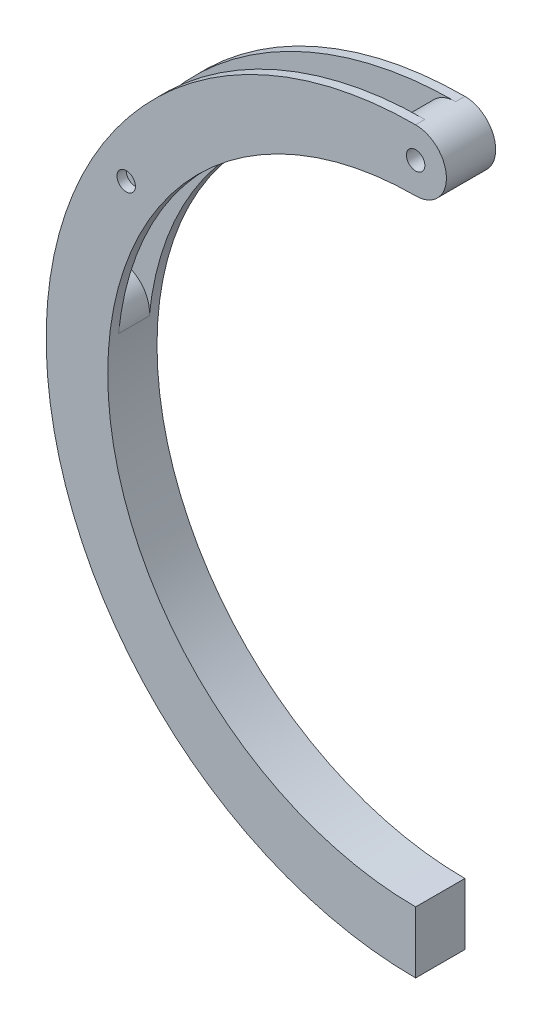
from build123d import *
from build123d.topology import SkipClean

# Parameters (mm, degrees)
FRONT_START                = 2.5
ARC_ARM_PROFILE_SKETCH_R   = 1.5
FRONT_ARC_PLATE_DEPTH      = 1.5
REAR_START                 = -2.5
SKETCH1_2_R                = 1.5
REAR_ARC_PLATE_DEPTH       = 1.5
END_SPACER_SKETCH_R        = 5
END_SPACER_SKETCH_R_2      = 1.5
END_SPACER_BLOCK_5MM_DEPTH = 5


with BuildPart() as part:
    # Arc Arm Profile Sketch → Front Arc Plate (new body)
    with BuildSketch(Plane.XY.offset(FRONT_START)):
        with BuildLine():
            Line((0, -50), (0, -60))
            ThreePointArc((0, -60), (-60, 0), (0, 60))
            ThreePointArc((0, 60), (5, 55), (0, 50))
            ThreePointArc((0, 50), (-50, 0), (0, -50))
        make_face()
        with Locations((0, 55)):
            Circle(ARC_ARM_PROFILE_SKETCH_R, mode=Mode.SUBTRACT)
        with Locations((-47, 28.565713714)):
            Circle(ARC_ARM_PROFILE_SKETCH_R, mode=Mode.SUBTRACT)
    extrude(amount=FRONT_ARC_PLATE_DEPTH)



with BuildPart() as body_2:
    # Sketch1_2 → Rear Arc Plate (new body)
    with BuildSketch(Plane.XY.offset(REAR_START)):
        with BuildLine():
            Line((0, -50), (0, -60))
            ThreePointArc((0, -60), (-60, 0), (0, 60))
            ThreePointArc((0, 60), (5, 55), (0, 50))
            ThreePointArc((0, 50), (-50, 0), (0, -50))
        make_face()
        with Locations((0, 55)):
            Circle(SKETCH1_2_R, mode=Mode.SUBTRACT)
        with Locations((-47, 28.565713714)):
            Circle(SKETCH1_2_R, mode=Mode.SUBTRACT)
    extrude(amount=-REAR_ARC_PLATE_DEPTH)


with BuildPart() as part_1:
    with SkipClean():  # the faces are left unmerged after this step: merging them gives an invalid solid
        add(part.part)

        add(body_2.part)  # End Spacer Block 5mm merges body 2
        # End Spacer Sketch → End Spacer Block 5mm (add)
        # profile 1 of 2: a face of its own
        with BuildSketch(Plane.XY.offset(-2.5)):
            with Locations(Location((0, 55, 0), (0, 0, 270))):
                Circle(END_SPACER_SKETCH_R)
            with Locations((0, 55)):
                Circle(END_SPACER_SKETCH_R_2, mode=Mode.SUBTRACT)
        # profile 2 of 2: a face of its own
        with BuildSketch(Plane.XY.offset(-2.5)):
            with BuildLine():
                Line((0, -60), (0, -50))
                ThreePointArc((0, -50), (-37.079584068, -33.542576606), (-49.749791564, 4.995822185))
                ThreePointArc((-49.749791564, 4.995822185), (-54.225188502, 10.47038356), (-59.699749877, 5.994986622))
                ThreePointArc((-59.699749877, 5.994986622), (-44.495500881, -40.251091927), (0, -60))
            make_face()
        extrude(amount=END_SPACER_BLOCK_5MM_DEPTH)


solid = part_1.part
